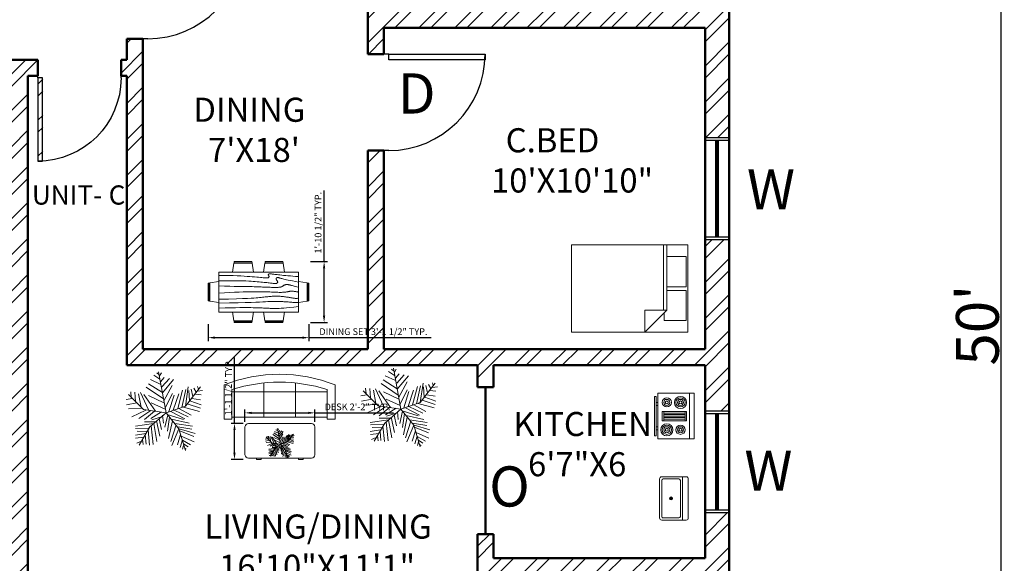
# Model space of a CAD drawing. Units: inches. Extents: x -31842 to -29388, y 18869 to 19743.
# Tile 8 of 12: x -30617 to -30250, y 19226 to 19429. Entities that reach past the tile are written whole.
import ezdxf

# ---------------------------------------------------------------- set-up
doc = ezdxf.new("R2010")
doc.units = ezdxf.units.IN
for name, color, linetype, lineweight in [('A-ANNO-DIMS', 2, 'Continuous', 18), ('A-ANNO-SYMB', 2, 'Continuous', 18), ('A-AREA-IDEN', 3, 'Continuous', 18), ('A-DOOR', 3, 'Continuous', 25), ('A-FLOR-FIXT', 8, 'Continuous', 18), ('A-FURN', 8, 'Continuous', 18), ('A-GLAZ', 4, 'Continuous', 25), ('A-WALL', 7, 'Continuous', 50), ('A-WALL-PATT', 8, 'Continuous', 13), ('L-PLNT', 3, 'Continuous', 13)]:
    doc.layers.add(name, color=color, linetype=linetype, lineweight=lineweight)
doc.styles.get("Standard").update_dxf_attribs({"font": 'arial.ttf'})
doc.dimstyles.new('ISO-25', dxfattribs={"dimtxt": 2.5, "dimasz": 2.5, "dimexe": 1.25, "dimexo": 0.625, "dimtad": 1, "dimdec": 0, "dimlunit": 3, "dimtxsty": 'Standard', "dimcen": 2.5, "dimadec": 0, "dimazin": 0, "dimtfac": 1, "dimtdec": 0, "dimtmove": 0, "dimatfit": 3, "dimfxl": 1, "dimarcsym": 0})

# ---------------------------------------------------------------- blocks, each defined once
blk = doc.blocks.new('*U8')
for p, q in [((0, 0), (0, -100)), ((750, 0), (750, -100))]:
    blk.add_line(p, q)
blk.add_lwpolyline([(0, 0), (0, 750), (43.75, 750), (43.75, 0)], close=True)
blk.add_arc((0, 0), 750, 0, 90)
blk = doc.blocks.new('Bed - Queen')
for p, q in [((0, -80.00003), (0, 0)), ((0, 0), (59.99999, 0)), ((59.99999, 0), (59.99999, -80.00003)), ((7.99999, -1.2), (28.79998, -1.2)), ((7.99999, -14.4), (7.99999, -1.2)), ((28.79998, -1.2), (28.79998, -14.4)), ((31.19999, -1.2), (51.99999, -1.2)), ((31.19999, -14.4), (31.19999, -1.2)), ((51.99999, -1.2), (51.99999, -16.4)), ((0, -14.4), (44.8, -14.4)), ((44.8, -16.8), (0, -16.8)), ((59.99999, -29.6), (44.8, -14.4)), ((44.8, -14.4), (44.8, -29.6)), ((51.99999, -16.4), (46.79936, -16.4)), ((44.8, -29.6), (59.99999, -29.6)), ((59.99999, -80.00003), (0, -80.00003))]:
    blk.add_line(p, q)
blk = doc.blocks.new('Range-Oven - 30 in top')
for p, q in [((0, -3), (30, -3)), ((12, -6), (18, -6)), ((13, -20), (13, -6)), ((14, -6), (14, -20)), ((15, -20), (15, -6)), ((16, -6), (16, -20)), ((17, -20), (17, -6)), ((6, -24), (6, -25)), ((8, -25), (8, -24)), ((18, -20), (12, -20)), ((22, -25), (22, -24)), ((24, -24), (24, -25))]:
    blk.add_line(p, q)
for points in [[(0, -24), (0, 0), (30, 0), (30, -24)], [(12, -21), (12, -5), (18, -5), (18, -21)], [(2, -26), (2, -25), (28, -25), (28, -26)]]:
    blk.add_lwpolyline(points, close=True)
for centre, radius in [((6, -9), 4), ((6, -9), 3), ((24, -9), 3), ((6, -9), 2), ((6, -9), 1), ((24, -9), 2), ((24, -9), 1), ((6, -18), 3), ((6, -18), 2), ((6, -18), 1), ((24, -18), 4), ((24, -18), 3), ((24, -18), 2), ((24, -18), 1)]:
    blk.add_circle(centre, radius)
blk = doc.blocks.new('Sink-single - 30 in top')
blk.add_line((-15, -3.999996), (15, -3.999996))
for points in [[(-13.5, 0), (13.5, 0)], [(-15, -18.499996), (-15, -1.5)], [(-13.5, -17.499996), (-13.5, -6.499996)], [(-12.5, -5.499996), (12.5, -5.499996)], [(13.5, -6.499996), (13.5, -17.499996)], [(15, -1.5), (15, -18.499996)], [(13.5, -19.999996), (-13.5, -19.999996)], [(12.5, -18.499996), (-12.5, -18.499996)]]:
    blk.add_lwpolyline(points)
for radius in [1, 0.5]:
    blk.add_circle((0, -11.999996), radius)
for centre, radius, start, end in [((-13.5, -1.5), 1.5, 90, 180), ((-12.5, -6.499996), 1, 90, 180), ((12.5, -6.499996), 1, 0, 90), ((13.5, -1.5), 1.5, 0, 90), ((-13.5, -18.499996), 1.5, 180, 270), ((-12.5, -17.499996), 1, 180, 270), ((12.5, -17.499996), 1, 270, 0), ((13.5, -18.499996), 1.5, 270, 0)]:
    blk.add_arc(centre, radius, start, end)
blk = doc.blocks.new('Desk - 30 x 60 in.')
for p, q in [((-26.999995, 0), (26.999995, 0)), ((-29.999995, -27), (-29.999995, -3)), ((29.999995, -3), (29.999995, -27)), ((26.999995, -30), (-26.999995, -30)), ((-20.000005, -30), (-20.000005, -31)), ((-20.000005, -31), (-16.000005, -31)), ((-16.000005, -31), (-16.000005, -30)), ((15.999995, -31), (15.999995, -30)), ((19.999995, -31), (15.999995, -31)), ((19.999995, -30), (19.999995, -31))]:
    blk.add_line(p, q)
for centre, start, end in [((-26.499995, -3.5), 98.1301, 171.8699), ((26.499995, -3.5), 8.130102, 81.8699), ((-26.499995, -26.5), 188.1301, 261.8699), ((26.499995, -26.5), 278.1301, 351.8699)]:
    blk.add_arc(centre, 3.535534, start, end)
blk = doc.blocks.new('Sofa - Roundback 7 ft.')
for p, q in [((-12.00002, -32.4421), (-12.00003, -6.5971)), ((11.99997, -32.4421), (11.99998, -6.5971)), ((-36.000027, -34), (-36.000027, -11.4696)), ((-35.999844, -13.3819), (35.9998, -13.3819)), ((35.99998, -34), (35.99998, -11.4696)), ((-36.000027, -32.4421), (35.99998, -32.4421))]:
    blk.add_line(p, q)
for points in [[(-36.000027, -34), (-42.000027, -34), (-42.000027, -8)], [(41.99998, -8), (41.99998, -34), (35.99998, -34)]]:
    blk.add_lwpolyline(points)
for centre, radius, start, end in [((0, -114.25), 114.25, 68.43141, 111.5686), ((-0.00001, -127.1968), 121.1968, 72.72033, 107.2797)]:
    blk.add_arc(centre, radius, start, end)
blk = doc.blocks.new('Dining Set - 36 x 72 in.')
for p, q in [((-22, 27.5), (-22.1562, 26.50042)), ((-22, 27.5), (-6, 27.5)), ((-5.8437, 26.49966), (-6, 27.5)), ((6, 27.5), (5.8438, 26.50042)), ((6, 27.5), (22, 27.5)), ((22.1563, 26.49966), (22, 27.5)), ((36, 18), (-36, 18)), ((-36, 18), (-36, -18)), ((-22.2343, 26.00059), (-23.4847, 17.99762)), ((-22.2304, 26), (-5.7608, 26)), ((-5.8416, 26.5), (-22.1534, 26.5)), ((-4.5152, 17.99762), (-5.7655, 25.99926)), ((5.7657, 26.00059), (4.5153, 17.99762)), ((5.7696, 26), (22.2392, 26)), ((22.1584, 26.5), (5.8466, 26.5)), ((23.4848, 17.99762), (22.2345, 25.99926)), ((36, -18), (36, 18)), ((-44.0006, 8.23428), (-35.9976, 9.48474)), ((44.0006, 8.23428), (35.9976, 9.48474)), ((-45.5, 8), (-44.5004, 8.15617)), ((-45.5, 8), (-45.5, -8)), ((-44.5, -8.15843), (-44.5, 8.15338)), ((-44, 8.23041), (-44, -8.23915)), ((44, 8.23041), (44, -8.23915)), ((44.5, -8.15843), (44.5, 8.15338)), ((45.5, 8), (44.5005, 8.15617)), ((45.5, 8), (45.5, -8)), ((-44.4997, -8.15631), (-45.5, -8)), ((-35.9976, -9.48476), (-43.9993, -8.2345)), ((35.9976, -9.48476), (43.9993, -8.2345)), ((44.4997, -8.15631), (45.5, -8)), ((-36, -18), (36, -18)), ((-22.2343, -26.0006), (-23.4847, -17.99762)), ((-22.2304, -26), (-5.7608, -26)), ((-22, -27.5), (-22.1562, -26.50044)), ((-5.8416, -26.5), (-22.1534, -26.5)), ((-5.8437, -26.49967), (-6, -27.5)), ((-4.5152, -17.99762), (-5.7655, -25.99928)), ((5.7657, -26.0006), (4.5153, -17.99762)), ((5.7696, -26), (22.2392, -26)), ((6, -27.5), (5.8438, -26.50044)), ((22.1584, -26.5), (5.8466, -26.5)), ((22.1563, -26.49967), (22, -27.5)), ((23.4848, -17.99762), (22.2345, -25.99928)), ((-22, -27.5), (-6, -27.5)), ((6, -27.5), (22, -27.5))]:
    blk.add_line(p, q)
for points in [[(-36, 15), (-31.1772, 14.97754), (-26.8079, 14.91406), (-22.8538, 14.81543), (-19.276, 14.6875), (-16.0362, 14.53613), (-13.0957, 14.36718), (-10.4159, 14.18652), (-7.9583, 14), (-5.6904, 13.81315), (-3.6035, 13.63021), (-1.6954, 13.45508), (0.0365, 13.29166), (1.5945, 13.14388), (2.9811, 13.01562), (4.1988, 12.9108), (5.25, 12.83333), (6.1393, 12.78613), (6.8802, 12.76823), (7.4883, 12.77767), (7.9792, 12.8125), (8.3685, 12.87077), (8.6719, 12.95052), (8.9049, 13.0498), (9.0833, 13.16666), (9.2205, 13.29899), (9.3216, 13.44401), (9.3895, 13.59879), (9.4271, 13.76041), (9.4373, 13.92594), (9.4232, 14.09245), (9.3875, 14.257), (9.3333, 14.41666), (9.2638, 14.56917), (9.1836, 14.71484), (9.0975, 14.85465), (9.0104, 14.98958), (8.9272, 15.1206), (8.8529, 15.2487), (8.7922, 15.37483), (8.75, 15.5), (8.7305, 15.62467), (8.7344, 15.74739), (8.7617, 15.86621), (8.8125, 15.97916), (8.8867, 16.08431), (8.9844, 16.17968), (9.1055, 16.26334), (9.25, 16.33333), (9.4189, 16.38802), (9.6172, 16.42708), (9.8506, 16.45052), (10.125, 16.45833), (10.4463, 16.45052), (10.8203, 16.42708), (11.2529, 16.38802), (11.75, 16.33333), (12.3184, 16.26318), (12.9694, 16.17838), (13.7151, 16.07991), (14.5677, 15.96875), (15.5395, 15.84586), (16.6426, 15.71224), (17.8893, 15.56884), (19.2917, 15.41666), (20.859, 15.25667), (22.5879, 15.08984), (24.4721, 14.91715), (26.5052, 14.73958), (28.6809, 14.5581), (30.9929, 14.3737), (33.4347, 14.18733), (36, 14)], [(-36, 10), (-28.9766, 10.14274), (-23.1725, 10.20442), (-18.4241, 10.19775), (-14.5677, 10.13541), (-11.4399, 10.03011), (-8.877, 9.89453), (-6.7154, 9.74137), (-4.7917, 9.58333), (-2.9698, 9.43082), (-1.2246, 9.28515), (0.4415, 9.14534), (2.026, 9.01041), (3.5266, 8.87939), (4.9408, 8.7513), (6.266, 8.62516), (7.5, 8.5), (8.6411, 8.37549), (9.6914, 8.2539), (10.6538, 8.13818), (11.5312, 8.03125), (12.3267, 7.93603), (13.043, 7.85547), (13.6831, 7.79248), (14.25, 7.75), (14.7471, 7.7303), (15.1797, 7.73307), (15.5537, 7.75732), (15.875, 7.80208), (16.1494, 7.86637), (16.3828, 7.94922), (16.5811, 8.04964), (16.75, 8.16666), (16.8944, 8.29915), (17.0143, 8.44531), (17.1089, 8.60319), (17.1771, 8.77083), (17.218, 8.94629), (17.2305, 9.1276), (17.2137, 9.31282), (17.1667, 9.5), (17.0895, 9.6875), (16.987, 9.875), (16.8649, 10.0625), (16.7292, 10.25), (16.5856, 10.4375), (16.4401, 10.625), (16.2985, 10.8125), (16.1667, 11), (16.05, 11.18733), (15.9518, 11.3737), (15.8752, 11.5581), (15.8229, 11.73958), (15.798, 11.91715), (15.8034, 12.08984), (15.842, 12.25667), (15.9167, 12.41666), (16.0295, 12.56836), (16.1784, 12.70833), (16.3605, 12.83268), (16.5729, 12.9375), (16.8127, 13.01888), (17.0768, 13.07291), (17.3625, 13.0957), (17.6667, 13.08333), (17.9894, 13.03312), (18.3418, 12.94726), (18.7382, 12.82918), (19.1927, 12.68229), (19.7195, 12.51001), (20.3327, 12.31575), (21.0465, 12.10294), (21.875, 11.875), (22.8357, 11.63354), (23.959, 11.37304), (25.2786, 11.08618), (26.8282, 10.76562), (28.6414, 10.40405), (30.752, 9.99414), (33.1936, 9.52856), (36, 9)], [(-36, 5.5), (-30.7157, 5.3348), (-26.069, 5.20963), (-21.9946, 5.11767), (-18.4271, 5.05208), (-15.3009, 5.00602), (-12.5508, 4.97265), (-10.1112, 4.94515), (-7.9167, 4.91666), (-5.909, 4.88167), (-4.0586, 4.83984), (-2.3429, 4.79215), (-0.7396, 4.73958), (0.7739, 4.6831), (2.22, 4.6237), (3.6213, 4.56233), (5, 4.5), (6.373, 4.43782), (7.7344, 4.3776), (9.0723, 4.32129), (10.375, 4.27083), (11.6309, 4.22819), (12.8281, 4.19531), (13.9551, 4.17415), (15, 4.16666), (15.954, 4.17448), (16.819, 4.19791), (17.6001, 4.23698), (18.3021, 4.29166), (18.9299, 4.36198), (19.4883, 4.44791), (19.9823, 4.54948), (20.4167, 4.66666), (20.7969, 4.79899), (21.1302, 4.94401), (21.4245, 5.09879), (21.6875, 5.26041), (21.9271, 5.42594), (22.1511, 5.59245), (22.3672, 5.757), (22.5834, 5.91666), (22.8065, 6.06868), (23.0404, 6.21093), (23.2879, 6.34147), (23.5521, 6.45833), (23.8358, 6.55957), (24.142, 6.64323), (24.4735, 6.70735), (24.8334, 6.75), (25.2235, 6.76969), (25.642, 6.76692), (26.0858, 6.74267), (26.5521, 6.69791), (27.0379, 6.63362), (27.5404, 6.55078), (28.0565, 6.45036), (28.5834, 6.33333), (29.1242, 6.19987), (29.7071, 6.04687), (30.3661, 5.87044), (31.1354, 5.66666), (32.0493, 5.43164), (33.142, 5.16146), (34.4475, 4.85221), (36, 4.5)], [(-36, -1), (-30.7915, -0.6591), (-26.0195, -0.38216), (-21.6519, -0.16284), (-17.6563, 0.00521), (-14.0005, 0.12833), (-10.6523, 0.21289), (-7.5796, 0.26522), (-4.75, 0.29166), (-2.134, 0.29793), (0.2878, 0.28711), (2.5317, 0.26163), (4.6146, 0.22396), (6.5529, 0.17651), (8.3633, 0.12174), (10.0623, 0.06209), (11.6667, 0), (13.1899, -0.06201), (14.6341, -0.1211), (15.9982, -0.17432), (17.2813, -0.21875), (18.4823, -0.25147), (19.6003, -0.26953), (20.6343, -0.27002), (21.5834, -0.25), (22.4481, -0.20768), (23.2357, -0.14584), (23.9549, -0.06836), (24.6146, 0.02083), (25.2235, 0.11784), (25.7904, 0.21875), (26.3241, 0.31966), (26.8334, 0.41666), (27.3265, 0.50618), (27.8099, 0.58593), (28.2894, 0.65397), (28.7709, 0.70833), (29.2601, 0.74707), (29.763, 0.76823), (30.2855, 0.76985), (30.8334, 0.75), (31.4088, 0.70784), (31.9994, 0.64713), (32.589, 0.57275), (33.1615, 0.48958), (33.7008, 0.4025), (34.1908, 0.3164), (34.6153, 0.23616), (34.9584, 0.16666), (35.2099, 0.11165), (35.3848, 0.07031), (35.504, 0.04069), (35.5886, 0.02083), (35.6594, 0.00879), (35.7377, 0.0026), (35.8442, 0.00032), (36, 0)], [(-36, -6.5), (-27.1843, -6.31267), (-20.084, -6.1263), (-14.469, -5.9419), (-10.1094, -5.76042), (-6.7752, -5.58285), (-4.2363, -5.41016), (-2.2629, -5.24333), (-0.625, -5.08334), (0.8708, -4.93099), (2.2715, -4.78646), (3.5872, -4.64974), (4.8281, -4.52084), (6.0046, -4.39974), (7.127, -4.28646), (8.2053, -4.18099), (9.25, -4.08334), (10.2705, -3.99382), (11.2734, -3.91407), (12.2647, -3.84603), (13.25, -3.79167), (14.2354, -3.75293), (15.2266, -3.73177), (16.2295, -3.73015), (17.25, -3.75), (18.2912, -3.79248), (19.3451, -3.85547), (20.4009, -3.93604), (21.4479, -4.03125), (22.4754, -4.13819), (23.4727, -4.25391), (24.4289, -4.37549), (25.3334, -4.5), (26.1785, -4.62492), (26.9694, -4.74935), (27.7145, -4.87281), (28.4219, -4.99479), (29.1, -5.11483), (29.7572, -5.23242), (30.4016, -5.34709), (31.0417, -5.45834), (31.6837, -5.56437), (32.3262, -5.65821), (32.9658, -5.73153), (33.599, -5.77604), (34.2224, -5.78345), (34.8327, -5.74545), (35.4264, -5.65373), (36, -5.5)], [(-36, -10), (-26.4022, -9.81299), (-18.4675, -9.62891), (-11.9839, -9.45069), (-6.7396, -9.28125), (-2.5226, -9.12354), (0.8789, -8.98047), (3.6769, -8.85498), (6.0833, -8.75), (8.2767, -8.66765), (10.3021, -8.60677), (12.1712, -8.56543), (13.8958, -8.54167), (15.4876, -8.53353), (16.9583, -8.53907), (18.3197, -8.55632), (19.5834, -8.58334), (20.7616, -8.61841), (21.8685, -8.66081), (22.9188, -8.71004), (23.9271, -8.76563), (24.9081, -8.82707), (25.8763, -8.89388), (26.8465, -8.96558), (27.8334, -9.04167), (28.8474, -9.12118), (29.8828, -9.20117), (30.93, -9.27824), (31.9792, -9.34896), (33.0205, -9.40991), (34.0443, -9.45768), (35.0407, -9.48885), (36, -9.5)], [(-36, -14.5), (-30.0881, -14.33513), (-25.0332, -14.21224), (-20.7312, -14.12647), (-17.0781, -14.07292), (-13.97, -14.04671), (-11.3027, -14.04297), (-8.9724, -14.05681), (-6.875, -14.08334), (-4.9224, -14.11833), (-3.0905, -14.16016), (-1.3709, -14.20785), (0.2448, -14.26042), (1.7647, -14.3169), (3.1973, -14.3763), (4.5507, -14.43767), (5.8333, -14.5), (7.0554, -14.5621), (8.235, -14.62175), (9.3922, -14.67652), (10.5469, -14.72396), (11.7192, -14.76164), (12.929, -14.78711), (14.1965, -14.79794), (15.5417, -14.79167), (16.9933, -14.76424), (18.6152, -14.70508), (20.4804, -14.60197), (22.6615, -14.44271), (25.2312, -14.21509), (28.2624, -13.9069), (31.8277, -13.50594), (36, -13)]]:
    blk.add_lwpolyline(points)
blk = doc.blocks.new('*U122')
for p, q in [((-258.7244, 1362.456), (-332.3336, 1421.4348)), ((0, 0), (-266.7, 1447.8)), ((-231.1146, 1315.2628), (-166.7002, 1421.4348)), ((-185.1152, 1008.5578), (-553.1612, 1185.4942)), ((-221.9198, 1197.3052), (-433.5526, 1338.8594)), ((-194.31, 1102.9442), (-65.4812, 1256.284)), ((-148.3106, 914.1968), (118.5418, 1220.9018)), ((-129.8956, 701.8528), (265.7602, 1185.4942)), ((-1234.059, 536.7274), (-1252.4486, 737.2604)), ((-1105.2302, 725.4494), (-1077.6458, 395.1732)), ((-902.8176, 713.6638), (-617.5756, 100.2538)), ((-93.091, 489.5342), (-700.3796, 902.3858)), ((-129.8956, 713.6638), (-626.7704, 1032.1544)), ((-74.7014, 418.7444), (219.7608, 961.39)), ((412.9786, 147.447), (587.8068, 796.2392)), ((560.197, 182.8292), (698.2206, 819.8358)), ((685.8, 228.6), (1219.2, 914.4)), ((689.0258, 230.0224), (790.2448, 914.1968)), ((808.6344, 784.4282), (827.0494, 418.7444)), ((891.4384, 831.6214), (946.658, 572.1096)), ((983.4626, 867.0036), (1066.2666, 725.4494)), ((1112.2914, 760.8316), (1296.3144, 784.4282)), ((1121.4862, 925.9824), (1149.0706, 831.6214)), ((-1206.4492, 501.3198), (-1418.082, 465.9376)), ((-800.1, 114.3), (-1333.5, 647.7)), ((-976.4268, 666.4706), (-884.4026, 194.6402)), ((-369.1382, 53.086), (-783.1836, 642.874)), ((-617.5756, 607.4918), (-74.7014, 347.98)), ((-28.6766, 171.0436), (228.9556, 678.2816)), ((100.1268, 41.275), (284.1498, 619.2774)), ((256.5654, 88.4682), (449.7832, 666.4706)), ((845.439, 418.7444), (1241.0948, 277.1902)), ((919.0482, 501.3198), (1222.6798, 454.152)), ((1029.462, 654.685), (1241.0948, 631.0884)), ((-1031.621, 347.98), (-1399.667, 277.1902)), ((-847.598, 159.2326), (-1326.0578, 135.636)), ((-718.7946, 88.4682), (-1215.644, -147.447)), ((-543.9664, 76.6572), (-967.2066, -206.4512)), ((0, 0), (-800.1, 114.3)), ((-405.9428, 53.086), (-764.794, -241.8334)), ((0, 0), (-571.5, -495.3)), ((-166.7002, 29.4894), (-543.9664, -206.4512)), ((-525.5514, 347.98), (-28.6766, 123.8504)), ((0, 0), (685.8, 228.6)), ((0, 0), (457.2, -571.5)), ((164.5412, 41.275), (661.416, -218.2368)), ((284.1498, 88.4682), (781.0246, -147.447)), ((458.978, 147.447), (891.4384, -88.4682)), ((615.4166, 194.6402), (1185.8752, 41.275)), ((753.4148, 312.5978), (1222.6798, 159.2326)), ((-387.5278, -324.4088), (-764.794, -324.4088)), ((-166.7002, -147.447), (-507.1618, -253.619)), ((-341.5284, -289.0012), (-221.9198, -831.6214)), ((-240.3094, -218.2368), (-157.5054, -595.7062)), ((-120.7008, -88.4682), (-93.091, -371.5766)), ((63.3222, -76.6826), (-37.8714, -513.1308)), ((44.9326, -64.897), (615.4166, -241.8334)), ((127.7366, -159.258), (54.1274, -654.685)), ((228.9556, -289.0012), (90.932, -914.1968)), ((192.151, -230.0224), (817.8292, -371.5766)), ((-442.7474, -383.3876), (-1086.8406, -477.7486)), ((-617.5756, -548.5384), (-1077.6458, -560.324)), ((-681.9646, -666.496), (-1022.4262, -654.685)), ((-571.5, -495.3), (-952.5, -1143)), ((-635.9652, -607.5172), (-580.771, -1150.1374)), ((-525.5514, -465.963), (-451.9422, -1126.5408)), ((-433.5526, -383.3876), (-323.1134, -1020.3688)), ((357.759, -430.5554), (164.5412, -1020.3688)), ((458.978, -572.1096), (210.5406, -1161.923)), ((311.7596, -383.3876), (937.4378, -477.7486)), ((412.9786, -501.3452), (919.0482, -583.9206)), ((457.2, -571.5), (685.8, -1333.5)), ((468.1982, -572.1096), (1029.462, -737.2604)), ((486.5878, -642.8994), (983.4626, -843.4324)), ((-718.7946, -737.2604), (-1086.8406, -796.2392)), ((-783.1836, -867.029), (-1077.6458, -902.4112)), ((-875.2078, -1008.5832), (-1040.8412, -1079.3476)), ((-829.2084, -937.7934), (-810.7934, -1126.5408)), ((-737.1842, -784.4536), (-709.5744, -1114.7298)), ((514.1976, -772.6426), (403.7838, -1138.3264)), ((578.612, -961.39), (495.7826, -1232.7128)), ((541.8074, -831.6214), (992.6574, -1032.1544)), ((578.612, -973.1756), (873.0488, -1138.3264)), ((624.6114, -1161.923), (587.8068, -1291.6916)), ((624.6114, -1102.9442), (781.0246, -1209.1162)), ((679.8056, -1268.095), (716.6102, -1291.6916))]:
    blk.add_line(p, q)
blk = doc.blocks.new('*D203')
at = {"layer": 'A-ANNO-DIMS', "color": 0, "lineweight": -2, "transparency": 16777216}
for p, q in [((-30351.77, 19614.99), (-30249.67, 19614.99)), ((-30250.92, 19612.49), (-30250.92, 19017.46)), ((-30351.77, 19014.96), (-30249.67, 19014.96))]:
    blk.add_line(p, q, dxfattribs=at)
at = {"layer": 'A-ANNO-DIMS', "color": 0, "transparency": 16777216}
for points in [[(-30251.34, 19612.49), (-30250.5, 19612.49), (-30250.92, 19614.99)], [(-30251.34, 19017.46), (-30250.5, 19017.46), (-30250.92, 19014.96)]]:
    blk.add_solid(points, dxfattribs=at)
at = {"layer": 'Defpoints', "color": 0, "transparency": 16777216}
for p in [(-30352.39, 19614.99), (-30352.39, 19014.96), (-30250.92, 19014.96)]:
    blk.add_point(p, dxfattribs=at)
at = {"layer": 'A-ANNO-DIMS', "color": 0, "transparency": 16777216, "insert": (-30259.72, 19314.97), "char_height": 2.5, "attachment_point": 5, "rotation": 90}
blk.add_mtext("{\\H6.4x;50'}", dxfattribs=at)
blk = doc.blocks.new('WIN-3FT')
for p, q in [((0, 36), (9, 36)), ((4, 0), (4, 36)), ((4.5, 0), (4.5, 36)), ((5, 0), (5, 36)), ((0, 0), (9, 0))]:
    blk.add_line(p, q)
blk = doc.blocks.new('*D243')
at = {"layer": 'A-ANNO-DIMS', "color": 0, "lineweight": -2, "transparency": 16777216}
for p, q in [((-30546.99, 19315.3), (-30546.99, 19309.03)), ((-30509.35, 19315.3), (-30509.35, 19309.03)), ((-30544.49, 19310.28), (-30511.85, 19310.28)), ((-30509.35, 19310.28), (-30463.71, 19310.28))]:
    blk.add_line(p, q, dxfattribs=at)
at = {"layer": 'A-ANNO-DIMS', "color": 0, "transparency": 16777216}
for points in [[(-30544.49, 19310.7), (-30544.49, 19309.86), (-30546.99, 19310.28)], [(-30511.85, 19310.7), (-30511.85, 19309.86), (-30509.35, 19310.28)]]:
    blk.add_solid(points, dxfattribs=at)
at = {"layer": 'Defpoints', "color": 0, "transparency": 16777216}
for p in [(-30546.99, 19315.93), (-30509.35, 19315.93), (-30509.35, 19310.28)]:
    blk.add_point(p, dxfattribs=at)
at = {"layer": 'A-ANNO-DIMS', "color": 0, "transparency": 16777216, "insert": (-30485.28, 19312.2), "char_height": 2.5, "attachment_point": 5}
blk.add_mtext('DINING SET 3\'-1 1/2" TYP.', dxfattribs=at)
blk = doc.blocks.new('*D244')
at = {"layer": 'A-ANNO-DIMS', "color": 0, "lineweight": -2, "transparency": 16777216}
for p, q in [((-30503.71, 19338.67), (-30503.71, 19365.2)), ((-30508.73, 19338.67), (-30502.46, 19338.67)), ((-30503.71, 19318.43), (-30503.71, 19336.17)), ((-30508.73, 19315.93), (-30502.46, 19315.93))]:
    blk.add_line(p, q, dxfattribs=at)
at = {"layer": 'A-ANNO-DIMS', "color": 0, "transparency": 16777216}
for points in [[(-30504.12, 19336.17), (-30503.29, 19336.17), (-30503.71, 19338.67)], [(-30504.12, 19318.43), (-30503.29, 19318.43), (-30503.71, 19315.93)]]:
    blk.add_solid(points, dxfattribs=at)
at = {"layer": 'Defpoints', "color": 0, "transparency": 16777216}
for p in [(-30509.35, 19338.67), (-30503.71, 19338.67), (-30509.35, 19315.93)]:
    blk.add_point(p, dxfattribs=at)
at = {"layer": 'A-ANNO-DIMS', "color": 0, "transparency": 16777216, "insert": (-30505.62, 19353.19), "char_height": 2.5, "attachment_point": 5, "rotation": 90}
blk.add_mtext('1\'-10 1/2" TYP.', dxfattribs=at)
blk = doc.blocks.new('*D249')
at = {"layer": 'A-ANNO-DIMS', "color": 0, "lineweight": -2, "transparency": 16777216}
for p, q in [((-30533.26, 19278.92), (-30533.26, 19283.46)), ((-30507.15, 19278.92), (-30507.15, 19283.46)), ((-30530.76, 19282.21), (-30509.65, 19282.21)), ((-30507.15, 19282.21), (-30477.8, 19282.21))]:
    blk.add_line(p, q, dxfattribs=at)
at = {"layer": 'A-ANNO-DIMS', "color": 0, "transparency": 16777216}
for points in [[(-30530.76, 19282.62), (-30530.76, 19281.79), (-30533.26, 19282.21)], [(-30509.65, 19282.62), (-30509.65, 19281.79), (-30507.15, 19282.21)]]:
    blk.add_solid(points, dxfattribs=at)
at = {"layer": 'Defpoints', "color": 0, "transparency": 16777216}
for p in [(-30507.15, 19282.21), (-30533.26, 19278.29), (-30507.15, 19278.29)]:
    blk.add_point(p, dxfattribs=at)
at = {"layer": 'A-ANNO-DIMS', "color": 0, "transparency": 16777216, "insert": (-30491.22, 19284.12), "char_height": 2.5, "attachment_point": 5}
blk.add_mtext('DESK 2\'-2" TYP.', dxfattribs=at)
blk = doc.blocks.new('*D250')
at = {"layer": 'A-ANNO-DIMS', "color": 0, "lineweight": -2, "transparency": 16777216}
for p, q in [((-30537.17, 19278.29), (-30537.17, 19302.87)), ((-30533.88, 19278.29), (-30538.42, 19278.29)), ((-30537.17, 19267.3), (-30537.17, 19275.79)), ((-30533.88, 19264.8), (-30538.42, 19264.8))]:
    blk.add_line(p, q, dxfattribs=at)
at = {"layer": 'A-ANNO-DIMS', "color": 0, "transparency": 16777216}
for points in [[(-30537.59, 19275.79), (-30536.76, 19275.79), (-30537.17, 19278.29)], [(-30537.59, 19267.3), (-30536.76, 19267.3), (-30537.17, 19264.8)]]:
    blk.add_solid(points, dxfattribs=at)
at = {"layer": 'Defpoints', "color": 0, "transparency": 16777216}
for p in [(-30537.17, 19278.29), (-30533.26, 19278.29), (-30533.26, 19264.8)]:
    blk.add_point(p, dxfattribs=at)
at = {"layer": 'A-ANNO-DIMS', "color": 0, "transparency": 16777216, "insert": (-30539.09, 19291.83), "char_height": 2.5, "attachment_point": 5, "rotation": 90}
blk.add_mtext('1\'-1 1/2" TYP.', dxfattribs=at)

msp = doc.modelspace()

# ---------------------------------------------------------------- hatches: boundary and pattern name
at = {"layer": 'A-WALL-PATT'}
h = msp.add_hatch(dxfattribs=at)
h.set_pattern_fill('ANSI32', color=256)
h.paths.add_polyline_path([(-30352.39, 19656.96), (-30487.39, 19656.96), (-30487.39, 19614.96), (-30510.39, 19614.96), (-30510.39, 19605.96), (-30487.39, 19605.96), (-30487.39, 19558.38), (-30481.39, 19558.38), (-30481.39, 19605.96), (-30469.68, 19605.96), (-30469.68, 19614.96), (-30481.39, 19614.96), (-30481.39, 19650.96), (-30361.39, 19650.96), (-30361.39, 19614.96), (-30445.68, 19614.96), (-30445.68, 19605.96), (-30361.39, 19605.96), (-30361.39, 19564.96), (-30352.39, 19564.96)])
h.paths.add_polyline_path([(-30548.39, 19614.96), (-30599.39, 19614.96), (-30599.39, 19605.96), (-30577.39, 19605.96), (-30577.39, 19457.87), (-30571.39, 19457.87), (-30571.39, 19491.96), (-30560.76, 19491.96), (-30560.76, 19497.96), (-30571.39, 19497.96), (-30571.39, 19605.96), (-30548.39, 19605.96)])
h.paths.add_polyline_path([(-30637.39, 19614.96), (-30688.39, 19614.96), (-30688.39, 19605.96), (-30665.39, 19605.96), (-30665.39, 19497.96), (-30682.48, 19497.96), (-30682.48, 19491.96), (-30665.39, 19491.96), (-30665.39, 19454.79), (-30662.43, 19454.79), (-30659.39, 19454.79), (-30659.39, 19605.96), (-30637.39, 19605.96)])
h.paths.add_polyline_path([(-30789.63, 19614.96), (-30875.39, 19614.96), (-30875.39, 19650.96), (-30755.39, 19650.96), (-30755.39, 19614.96), (-30765.63, 19614.96), (-30765.63, 19605.96), (-30755.39, 19605.96), (-30755.39, 19550.68), (-30749.39, 19550.68), (-30749.39, 19605.96), (-30726.39, 19605.96), (-30726.39, 19614.96), (-30749.39, 19614.96), (-30749.39, 19656.96), (-30884.39, 19656.96), (-30884.39, 19564.96), (-30875.39, 19564.96), (-30875.39, 19605.96), (-30789.63, 19605.96)])
h.paths.add_polyline_path([(-30749.39, 19491.96), (-30736.92, 19491.96), (-30736.92, 19494.96), (-30682.48, 19494.96), (-30682.48, 19497.96), (-30665.39, 19497.96), (-30665.39, 19605.96), (-30688.39, 19605.96), (-30749.39, 19605.96), (-30749.39, 19550.68), (-30755.39, 19550.68), (-30757.34, 19550.71, 0.39722), (-30793.34, 19516.76), (-30757.34, 19516.76), (-30757.34, 19514.65), (-30793.4, 19514.65), (-30793.4, 19516.76), (-30793.34, 19516.76, -0.39722), (-30757.34, 19550.71), (-30755.39, 19550.71), (-30755.39, 19605.96), (-30765.63, 19605.96), (-30765.63, 19613.66), (-30767.03, 19613.66), (-30767.03, 19637.62, 0.397344), (-30789.63, 19613.65), (-30789.63, 19605.96), (-30875.39, 19605.96), (-30875.39, 19564.96), (-30875.39, 19485.96), (-30873.79, 19485.96), (-30873.79, 19479.96), (-30873.79, 19479.35, 0.39722), (-30851.19, 19455.39), (-30851.19, 19479.35), (-30849.79, 19479.35), (-30849.79, 19455.34), (-30851.19, 19455.34), (-30851.19, 19455.39, -0.39722), (-30873.79, 19479.35), (-30873.79, 19479.96), (-30875.39, 19479.96), (-30875.39, 19431.96), (-30848.39, 19431.96), (-30848.39, 19468.96), (-30842.39, 19468.96), (-30842.39, 19479.96), (-30755.39, 19479.96), (-30755.39, 19470.97), (-30749.39, 19470.97)])
h.paths.add_polyline_path([(-30738.39, 19585.51), (-30738.39, 19586.08), (-30736.12, 19586.08), (-30736.12, 19586.65), (-30739.53, 19586.65), (-30739.53, 19600.27), (-30722.5, 19600.27), (-30722.5, 19586.65), (-30725.91, 19586.65), (-30725.91, 19586.08), (-30723.64, 19586.08), (-30723.64, 19585.51)], flags=16)
h.paths.add_polyline_path([(-30737.83, 19590.05, -1), (-30734.42, 19590.05, -1)], flags=16)
h.paths.add_polyline_path([(-30737.26, 19590.05, -1), (-30734.99, 19590.05, -1)], flags=0)
h.paths.add_polyline_path([(-30732.72, 19588.35), (-30732.72, 19597.43), (-30729.31, 19597.43), (-30729.31, 19588.35)], flags=16)
h.paths.add_polyline_path([(-30736.69, 19590.05, -1), (-30735.56, 19590.05, -1)], flags=0)
h.paths.add_polyline_path([(-30732.15, 19588.92), (-30732.15, 19596.86), (-30729.88, 19596.86), (-30729.88, 19588.92)], flags=0)
h.paths.add_polyline_path([(-30728.18, 19590.05, -1), (-30723.64, 19590.05, -1)], flags=0)
h.paths.add_polyline_path([(-30727.61, 19590.05, -1), (-30724.2, 19590.05, -1)], flags=0)
h.paths.add_polyline_path([(-30727.04, 19590.05, -1), (-30724.77, 19590.05, -1)], flags=0)
h.paths.add_polyline_path([(-30726.47, 19590.05, -1), (-30725.34, 19590.05, -1)], flags=0)
h.paths.add_polyline_path([(-30738.39, 19595.16, -1), (-30733.85, 19595.16, -1)], flags=16)
h.paths.add_polyline_path([(-30737.83, 19595.16, -1), (-30734.42, 19595.16, -1)], flags=0)
h.paths.add_polyline_path([(-30737.26, 19595.16, -1), (-30734.99, 19595.16, -1)], flags=0)
h.paths.add_polyline_path([(-30736.69, 19595.16, -1), (-30735.56, 19595.16, -1)], flags=0)
h.paths.add_polyline_path([(-30727.61, 19595.16, -1), (-30724.2, 19595.16, -1)], flags=0)
h.paths.add_polyline_path([(-30727.04, 19595.16, -1), (-30724.77, 19595.16, -1)], flags=0)
h.paths.add_polyline_path([(-30707.55, 19587.34, -0.414214), (-30708.36, 19588.14), (-30708.36, 19597.29, -0.414214), (-30707.55, 19598.09), (-30693.03, 19598.09, -0.414214), (-30692.23, 19597.29), (-30692.23, 19588.14, -0.414214), (-30693.03, 19587.34)], flags=16)
h.paths.add_polyline_path([(-30726.47, 19595.16, -1), (-30725.34, 19595.16, -1)], flags=0)
h.paths.add_polyline_path([(-30827.74, 19570.11), (-30871.22, 19570.11), (-30871.22, 19602.72), (-30827.74, 19602.72)], flags=16)
h.paths.add_polyline_path([(-30707.01, 19588.14, -0.414214), (-30707.55, 19588.68), (-30707.55, 19594.6, -0.414214), (-30707.01, 19595.13), (-30693.57, 19595.13, -0.414214), (-30693.03, 19594.6), (-30693.03, 19588.68, -0.414214), (-30693.57, 19588.14)], flags=0)
h.paths.add_polyline_path([(-30700.02, 19591.64, -1), (-30700.56, 19591.64, -1)], flags=0)
h.paths.add_polyline_path([(-30863.39, 19594.46), (-30863.39, 19574.46), (-30870.57, 19574.46), (-30870.57, 19585.76), (-30863.39, 19585.76), (-30863.39, 19587.07), (-30870.57, 19587.07), (-30870.57, 19598.37), (-30862.31, 19598.37), (-30862.31, 19595.55), (-30855.13, 19602.72), (-30855.13, 19594.46)], flags=0)
h.paths.add_polyline_path([(-30755.39, 19514.65), (-30757.34, 19514.65), (-30793.4, 19514.65), (-30793.4, 19516.76), (-30793.34, 19516.76, -0.39722), (-30757.34, 19550.71), (-30755.39, 19550.71), (-30755.39, 19605.96), (-30765.63, 19605.96), (-30765.63, 19613.66), (-30767.03, 19613.66), (-30767.03, 19637.62, 0.397344), (-30789.63, 19613.65), (-30789.63, 19605.96), (-30875.39, 19605.96), (-30875.39, 19564.96), (-30875.39, 19485.96), (-30873.79, 19485.96), (-30873.79, 19479.96), (-30873.79, 19479.35, 0.39722), (-30851.19, 19455.39), (-30851.19, 19479.35), (-30849.79, 19479.35), (-30849.79, 19479.96), (-30849.79, 19479.96), (-30849.79, 19485.96), (-30755.39, 19485.96)], flags=16)
h.paths.add_polyline_path([(-30665.39, 19605.96), (-30688.39, 19605.96), (-30749.39, 19605.96), (-30749.39, 19550.68), (-30755.39, 19550.68), (-30757.34, 19550.71, 0.39722), (-30793.34, 19516.76), (-30757.34, 19516.76), (-30757.34, 19514.65), (-30755.39, 19514.65), (-30755.39, 19514.68), (-30749.39, 19514.68), (-30749.39, 19497.96), (-30736.92, 19497.96), (-30736.92, 19494.96), (-30682.48, 19494.96), (-30682.48, 19497.96), (-30665.39, 19497.96)], flags=17)
h.paths.add_polyline_path([(-30749.39, 19446.97), (-30755.39, 19446.97), (-30755.39, 19431.96), (-30842.39, 19431.96), (-30842.39, 19442.96), (-30848.39, 19442.96), (-30848.39, 19431.96), (-30875.39, 19431.96), (-30875.39, 19479.96), (-30873.79, 19479.96), (-30873.79, 19482.55), (-30873.79, 19485.96), (-30875.39, 19485.96), (-30875.39, 19526.96), (-30884.39, 19526.96), (-30884.39, 19384.96), (-30875.39, 19384.96), (-30875.39, 19425.96), (-30755.39, 19425.96), (-30755.39, 19414.67), (-30751.3, 19414.67), (-30749.39, 19414.62)])
h.paths.add_polyline_path([(-30848.39, 19468.96), (-30848.39, 19479.96), (-30849.79, 19479.96), (-30849.79, 19479.35), (-30849.79, 19455.34), (-30851.19, 19455.34), (-30851.19, 19455.39, -0.39722), (-30873.79, 19479.35), (-30873.79, 19479.96), (-30875.39, 19479.96), (-30875.39, 19431.96), (-30848.39, 19431.96), (-30848.39, 19442.96)], flags=17)
h.paths.add_polyline_path([(-30659.39, 19407.96), (-30657.22, 19407.96), (-30657.22, 19413.96), (-30659.39, 19413.96), (-30659.39, 19418.79), (-30665.39, 19418.79), (-30665.39, 19305.96), (-30749.39, 19305.96), (-30749.39, 19378.62), (-30755.39, 19378.62), (-30755.39, 19305.96), (-30875.39, 19305.96), (-30875.39, 19346.96), (-30884.39, 19346.96), (-30884.39, 19282.96), (-30875.39, 19282.96), (-30875.39, 19299.96), (-30796.39, 19299.96), (-30796.39, 19286.68), (-30790.39, 19286.68), (-30790.39, 19299.96), (-30659.39, 19299.96)])
h.paths.add_polyline_path([(-30352.39, 19346.96), (-30361.39, 19346.96), (-30361.39, 19305.96), (-30481.39, 19305.96), (-30481.39, 19380.1), (-30487.39, 19380.1), (-30487.39, 19305.96), (-30571.39, 19305.96), (-30571.39, 19421.87), (-30577.39, 19421.87), (-30577.39, 19413.96), (-30579.53, 19413.96), (-30579.53, 19407.96), (-30577.39, 19407.96), (-30577.39, 19299.96), (-30446.39, 19299.96), (-30446.39, 19291.76), (-30440.39, 19291.76), (-30440.39, 19299.96), (-30361.39, 19299.96), (-30361.39, 19282.96), (-30352.39, 19282.96)])
h.paths.add_polyline_path([(-30481.39, 19449.62), (-30484.39, 19449.62), (-30487.39, 19449.62), (-30487.39, 19416.1), (-30481.39, 19416.1), (-30481.39, 19425.96), (-30361.39, 19425.96), (-30361.39, 19384.96), (-30352.39, 19384.96), (-30352.39, 19526.96), (-30361.39, 19526.96), (-30361.39, 19485.96), (-30363.32, 19485.96), (-30363.32, 19479.96), (-30361.39, 19479.96), (-30361.39, 19431.96), (-30388.39, 19431.96), (-30388.39, 19442.96), (-30394.39, 19442.96), (-30394.39, 19431.96), (-30481.39, 19431.96)])
h.paths.add_polyline_path([(-30387.32, 19482.76), (-30387.32, 19485.96), (-30481.39, 19485.96), (-30481.39, 19522.38), (-30487.39, 19522.38), (-30487.39, 19497.96), (-30500.08, 19497.96), (-30500.08, 19491.96), (-30487.39, 19491.96), (-30487.39, 19473.62), (-30481.39, 19473.62), (-30481.39, 19479.96), (-30394.39, 19479.96), (-30394.39, 19468.96), (-30388.39, 19468.96), (-30388.39, 19479.96), (-30387.32, 19479.96)])
h.paths.add_polyline_path([(-30626.04, 19413.96), (-30610.58, 19413.96), (-30610.58, 19407.24), (-30608.81, 19407.24), (-30608.81, 19376.14), (-30610.63, 19376.14), (-30610.63, 19407.96), (-30614.39, 19407.96), (-30614.39, 19173.96), (-30532.79, 19173.96), (-30532.79, 19167.96), (-30532.79, 19166.59), (-30532.79, 19167.96), (-30614.39, 19167.96), (-30614.39, 19023.96), (-30568.89, 19023.96), (-30568.89, 19014.96), (-30666.89, 19014.96), (-30666.89, 19018.96), (-30702.89, 19018.96), (-30702.89, 19019.96), (-30666.89, 19019.96), (-30666.89, 19023.96), (-30620.39, 19023.96), (-30620.39, 19167.96), (-30707.45, 19167.96), (-30707.45, 19166.65, -0.39722), (-30741.49, 19130.57), (-30741.49, 19130.51), (-30743.6, 19130.51), (-30743.6, 19166.65), (-30741.49, 19166.65), (-30741.49, 19130.57, 0.407721), (-30707.48, 19167.96), (-30707.53, 19167.96), (-30707.53, 19173.96), (-30620.39, 19173.96), (-30620.39, 19407.96), (-30626.04, 19407.96), (-30626.04, 19406.62), (-30626.04, 19375.45), (-30627.86, 19375.45), (-30627.86, 19406.62), (-30626.04, 19406.62), (-30626.04, 19407.96), (-30626.04, 19407.96)])
h.paths.add_polyline_path([(-30481.39, 19167.96), (-30478.24, 19167.96), (-30478.24, 19173.96), (-30487.39, 19173.96), (-30496.79, 19173.96), (-30496.79, 19167.96), (-30487.39, 19167.96), (-30487.39, 19023.96), (-30531.89, 19023.96), (-30531.89, 19014.96), (-30449.39, 19014.96), (-30449.39, 19023.96), (-30481.39, 19023.96)])
h.paths.add_polyline_path([(-30322.39, 19173.96), (-30343.77, 19173.96), (-30343.77, 19167.96), (-30328.39, 19167.96), (-30328.39, 19023.96), (-30373.39, 19023.96), (-30373.39, 19076.96), (-30379.39, 19076.96), (-30379.39, 19023.96), (-30411.39, 19023.96), (-30411.39, 19014.96), (-30322.39, 19014.96)])
h.paths.add_polyline_path([(-30367.77, 19173.96), (-30440.39, 19173.96), (-30440.39, 19191.96), (-30446.39, 19191.96), (-30446.39, 19173.96), (-30449.24, 19173.96), (-30449.24, 19167.96), (-30379.39, 19167.96), (-30379.39, 19114.96), (-30373.39, 19114.96), (-30373.39, 19167.96), (-30367.77, 19167.96)])
h.paths.add_polyline_path([(-30857.39, 19167.96), (-30814.74, 19167.96), (-30787.91, 19167.96), (-30787.91, 19173.96), (-30790.39, 19173.96), (-30790.39, 19191.02), (-30796.39, 19191.02), (-30796.39, 19173.96), (-30814.74, 19173.96), (-30871.78, 19173.96), (-30871.78, 19167.96), (-30863.39, 19167.96), (-30863.39, 19114.96), (-30857.39, 19114.96)])
h.paths.add_polyline_path([(-30857.39, 19076.96), (-30863.39, 19076.96), (-30863.39, 19023.96), (-30908.39, 19023.96), (-30908.39, 19167.96), (-30895.78, 19167.96), (-30895.78, 19173.96), (-30914.39, 19173.96), (-30914.39, 19014.96), (-30825.39, 19014.96), (-30825.39, 19023.96), (-30857.39, 19023.96)])
h.paths.add_polyline_path([(-30758.91, 19173.96), (-30743.53, 19173.96), (-30743.53, 19167.96), (-30743.6, 19166.65), (-30741.49, 19166.65), (-30741.49, 19130.51), (-30743.6, 19130.51), (-30743.6, 19166.65), (-30743.6, 19167.96), (-30749.39, 19167.96), (-30749.39, 19023.96), (-30702.89, 19023.96), (-30702.89, 19019.46), (-30666.89, 19019.46), (-30666.89, 19018.96), (-30702.89, 19018.96), (-30702.89, 19014.96), (-30788.39, 19014.96), (-30788.39, 19018.96), (-30824.39, 19018.96), (-30824.39, 19019.96), (-30788.39, 19019.96), (-30788.39, 19023.96), (-30755.39, 19023.96), (-30755.39, 19167.96), (-30758.91, 19167.96), (-30758.91, 19166.97), (-30758.91, 19137.97), (-30760.6, 19137.97), (-30760.6, 19166.97), (-30758.91, 19166.97), (-30758.91, 19167.96), (-30758.91, 19167.96)])
h.paths.add_polyline_path([(-30790.39, 19237.4), (-30796.39, 19237.4), (-30796.39, 19227.96), (-30875.39, 19227.96), (-30875.39, 19244.96), (-30884.39, 19244.96), (-30884.39, 19210.96), (-30875.39, 19210.96), (-30875.39, 19221.96), (-30796.39, 19221.96), (-30796.39, 19215.02), (-30793.87, 19215.02), (-30790.39, 19215.02)])
h.paths.add_polyline_path([(-30352.39, 19244.96), (-30361.39, 19244.96), (-30361.39, 19227.96), (-30440.39, 19227.96), (-30440.39, 19236.96), (-30446.39, 19236.96), (-30446.39, 19215.96), (-30440.39, 19215.96), (-30440.39, 19221.96), (-30361.39, 19221.96), (-30361.39, 19210.96), (-30352.39, 19210.96)])
h.paths.add_polyline_path([(-30788.99, 19602.36), (-30766.36, 19602.36), (-30766.36, 19633.27), (-30788.99, 19633.27)], flags=24)
h.paths.add_polyline_path([(-30871.43, 19460.05), (-30848.8, 19460.05), (-30848.8, 19490.96), (-30871.43, 19490.96)], flags=24)
h.paths.add_polyline_path([(-30778.82, 19519.23), (-30756.18, 19519.23), (-30756.18, 19550.14), (-30778.82, 19550.14)], flags=24)
h.paths.add_polyline_path([(-30741.54, 19533.68), (-30681.86, 19533.68), (-30681.86, 19567.23), (-30741.54, 19567.23)], flags=24)
h.paths.add_polyline_path([(-30866.65, 19526.15), (-30802.54, 19526.15), (-30802.54, 19559.73), (-30866.65, 19559.73)], flags=8)

# ---------------------------------------------------------------- linework, layer by layer
at = {"layer": 'A-GLAZ'}
for p, q in [((-30361.39, 19384.96), (-30352.39, 19384.96)), ((-30361.39, 19346.96), (-30352.39, 19346.96)), ((-30361.39, 19282.96), (-30352.39, 19282.96)), ((-30361.39, 19244.96), (-30352.39, 19244.96))]:
    msp.add_line(p, q, dxfattribs=at)
at = {"layer": 'A-WALL'}
for p, q in [((-30352.39, 19656.96), (-30352.39, 19173.96)), ((-30487.39, 19449.62), (-30487.39, 19416.1)), ((-30481.39, 19425.96), (-30361.39, 19425.96)), ((-30481.39, 19425.96), (-30481.39, 19416.1)), ((-30361.39, 19425.96), (-30361.39, 19305.96)), ((-30577.39, 19421.87), (-30571.39, 19421.87)), ((-30577.39, 19421.87), (-30577.39, 19413.96)), ((-30571.39, 19421.87), (-30571.39, 19305.96)), ((-30487.39, 19416.1), (-30481.39, 19416.1)), ((-30626.04, 19413.96), (-30610.58, 19413.96)), ((-30610.58, 19407.96), (-30610.58, 19413.96)), ((-30579.53, 19407.96), (-30579.53, 19413.96)), ((-30579.53, 19413.96), (-30577.39, 19413.96)), ((-30614.39, 19173.96), (-30614.39, 19407.96)), ((-30614.39, 19407.96), (-30610.58, 19407.96)), ((-30579.53, 19407.96), (-30577.39, 19407.96)), ((-30577.39, 19407.96), (-30577.39, 19299.96)), ((-30487.39, 19380.1), (-30481.39, 19380.1)), ((-30487.39, 19380.1), (-30487.39, 19305.96)), ((-30481.39, 19380.1), (-30481.39, 19305.96)), ((-30571.39, 19305.96), (-30487.39, 19305.96)), ((-30481.39, 19305.96), (-30361.39, 19305.96)), ((-30577.39, 19299.96), (-30446.39, 19299.96)), ((-30446.39, 19299.96), (-30446.39, 19291.76)), ((-30440.39, 19299.96), (-30440.39, 19291.76)), ((-30440.39, 19299.96), (-30361.39, 19299.96)), ((-30361.39, 19299.96), (-30361.39, 19227.96)), ((-30446.39, 19291.76), (-30440.39, 19291.76)), ((-30443.39, 19291.76), (-30443.39, 19236.96)), ((-30446.39, 19236.96), (-30440.39, 19236.96)), ((-30446.39, 19236.96), (-30446.39, 19215.96)), ((-30440.39, 19236.96), (-30440.39, 19227.96)), ((-30440.39, 19227.96), (-30361.39, 19227.96))]:
    msp.add_line(p, q, dxfattribs=at)

# ---------------------------------------------------------------- block references
at = {"layer": 'A-DOOR'}
for p, xscale, yscale, zscale, rotation in [((-30569.59, 19457.87), 0.0479999960937841, 0.0479999960937841, 0.0479999960937841, 270), ((-30479.59, 19416.1), 0.0479999960937836, 0.0479999960937836, 0.0479999960937836, 270), ((-30610.63, 19407.24), -0.0414596924890394, 0.0414596924890394, 0.0414596924890394, 180)]:
    msp.add_blockref('*U8', p, dxfattribs=dict(at, xscale=xscale, yscale=yscale, zscale=zscale, rotation=rotation))
at = {"layer": 'A-FLOR-FIXT', "rotation": 270}
for name, p, xscale, yscale, zscale in [('Range-Oven - 30 in top', (-30365.5, 19289.51), 0.5676462121975467, 0.5676462121975467, 0.5676462121975467), ('Sink-single - 30 in top', (-30367.68, 19250.27), 0.5377581895364227, 0.5377581895364227, 0.5377581895364227)]:
    msp.add_blockref(name, p, dxfattribs=dict(at, xscale=xscale, yscale=yscale, zscale=zscale))
at = {"layer": 'A-FURN', "xscale": 0.5435212084103092, "yscale": 0.5435212084103092, "zscale": 0.5435212084103092, "rotation": 270}
msp.add_blockref('Bed - Queen', (-30367.84, 19344.89), dxfattribs=at)
at = {"layer": 'A-FURN'}
for name, p, xscale, yscale, zscale in [('Dining Set - 36 x 72 in.', (-30528.17, 19327.3), 0.4136315660595786, 0.4136315660595786, 0.4136315660595786), ('Sofa - Roundback 7 ft.', (-30520.35, 19296.61), 0.4932806057472628, 0.4932806057472628, 0.4932806057472628), ('Desk - 30 x 60 in.', (-30520.2, 19278.29), 0.435161060015466, 0.435161060015466, 0.435161060015466)]:
    msp.add_blockref(name, p, dxfattribs=dict(at, xscale=xscale, yscale=yscale, zscale=zscale))
at = {"layer": 'A-GLAZ'}
for p in [(-30361.39, 19347.96), (-30361.39, 19245.96)]:
    msp.add_blockref('WIN-3FT', p, dxfattribs=at)
at = {"layer": 'L-PLNT'}
for p, xscale, yscale, zscale in [((-30475.04, 19283.61), 0.0105251743607086, 0.0105251743607086, 0.0105251743607086), ((-30562.74, 19282.24), 0.0105251743607086, 0.0105251743607086, 0.0105251743607086), ((-30520.01, 19270.57), 0.0039973248373877, 0.0039973248373877, 0.0039973248373877)]:
    msp.add_blockref('*U122', p, dxfattribs=dict(at, xscale=xscale, yscale=yscale, zscale=zscale))

# ---------------------------------------------------------------- texts
at = {"layer": 'A-ANNO-SYMB', "char_height": 15, "attachment_point": 1}
for s, insert in [('{D}', (-30476.16, 19408.93)), ('{W}', (-30345.79, 19373.12)), ('{W}', (-30346.75, 19268.12)), ('{O}', (-30442.05, 19262.24))]:
    msp.add_mtext_dynamic_manual_height_columns(s, width=971.0743, gutter_width=12.5, heights=[0], dxfattribs=dict(at, insert=insert))
at = {"layer": 'A-AREA-IDEN', "attachment_point": 1}
for s, width, insert, char_height in [("{DINING\\P  7'X18'}", 1016.678, (-30552.55, 19399.85), 9), ('{   C.BED\\P 10\'X10\'10"}', 1016.678, (-30444.14, 19388.45), 9), ('{UNIT-^IC}', 971.0743, (-30612.84, 19367.11), 7.168), ('{KITCHEN\\P  6\'7"X6}', 1016.678, (-30433.04, 19282.54), 9), ('{LIVING/DINING\\P  16\'10"X11\'1"}', 1016.678, (-30548.42, 19244.27), 9)]:
    msp.add_mtext_dynamic_manual_height_columns(s, width=width, gutter_width=12.5, heights=[0], dxfattribs=dict(at, insert=insert, char_height=char_height))

# ---------------------------------------------------------------- dimensions: what is measured, and where the dimension line sits
at = {"layer": 'A-ANNO-DIMS'}
for base, p1, p2, text, override, picture, middle in [((-30250.92, 19014.96), (-30352.39, 19614.99), (-30352.39, 19014.96), '{\\H6.4x;<>}', {"dimclrd": 0, "dimclre": 0, "dimclrt": 0}, '*D203', (-30259.72, 19314.97)), ((-30503.71, 19338.67), (-30509.35, 19315.93), (-30509.35, 19338.67), '<> TYP.', {"dimdec": 1, "dimlfac": 1, "dimrnd": 0, "dimzin": 1, "dimdsep": 46, "dimlunit": 4, "dimfrac": 2}, '*D244', (-30505.62, 19353.19)), ((-30537.17, 19278.29), (-30533.26, 19264.8), (-30533.26, 19278.29), '<> TYP.', {"dimdec": 1, "dimlfac": 1, "dimrnd": 0, "dimzin": 1, "dimdsep": 46, "dimlunit": 4, "dimfrac": 2}, '*D250', (-30539.09, 19291.83))]:
    dim = msp.add_linear_dim(base=base, p1=p1, p2=p2, angle=90, text=text, dimstyle='ISO-25', override=override, dxfattribs=at)
    dim.commit()
    dim.dimension.update_dxf_attribs({"geometry": picture, "text_midpoint": middle})
for base, p1, p2, text, picture, middle in [((-30509.35, 19310.28), (-30546.99, 19315.93), (-30509.35, 19315.93), 'DINING SET <> TYP.', '*D243', (-30485.28, 19312.2)), ((-30507.15, 19282.21), (-30533.26, 19278.29), (-30507.15, 19278.29), 'DESK <> TYP.', '*D249', (-30491.22, 19284.12))]:
    dim = msp.add_linear_dim(base=base, p1=p1, p2=p2, text=text, dimstyle='ISO-25', override={"dimdec": 1, "dimlfac": 1, "dimrnd": 0, "dimzin": 1, "dimdsep": 46, "dimlunit": 4, "dimfrac": 2}, dxfattribs=at)
    dim.commit()
    dim.dimension.update_dxf_attribs({"geometry": picture, "text_midpoint": middle})

doc.saveas('drawing.dxf')
